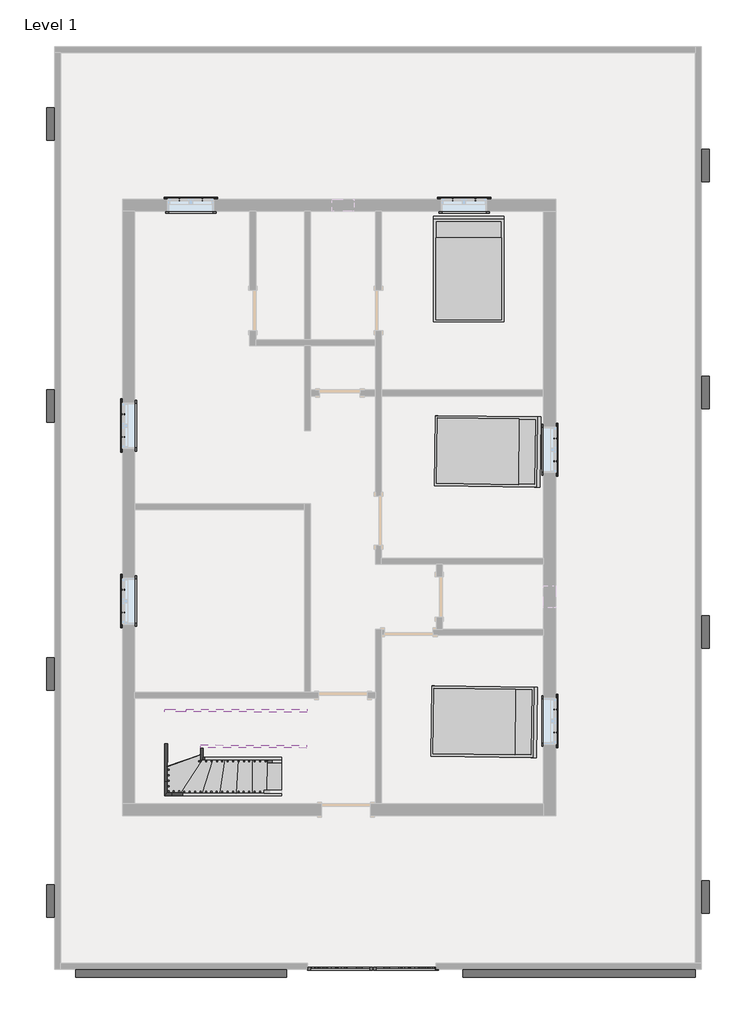
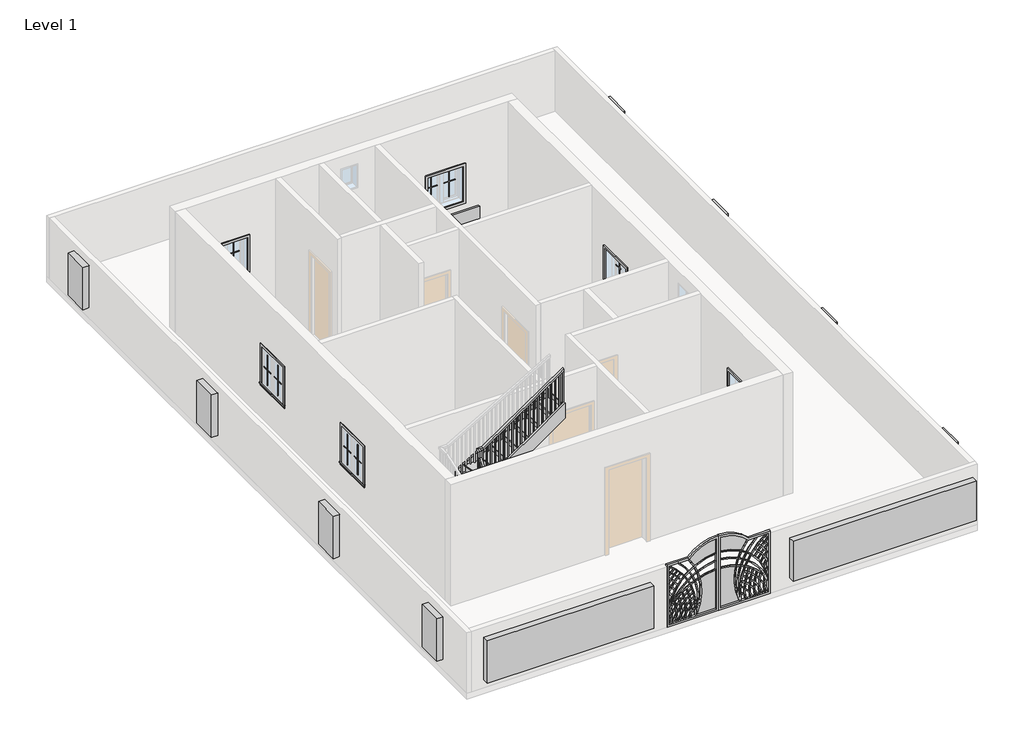
# One storey, part 3 of 3: 28 proxies, 9 members, 3 furniture elements, 1 railing, 1 stair flight.
"""IFC4 building model written with IfcOpenShell, lengths in millimetres."""

from ifc_helpers import new_model, si_unit, frame, origin, place, context, project, spatial, polyline, outline, extrude, faceted_brep, transform, mapped, element, save
from components import generic_models_6bc30956, generic_models_1_generic_models_1_75855b24, generic_models_2_generic_models_2_0c6c8571, generic_models_3_generic_models_3_96fd7fd6, muntin_pattern_2x2_muntin_pattern_2x2_b3fe6957, muntin_pattern_2x2_muntin_pattern_2x2_3e0ecaf2, trim_window_exterior_flat_with_sill_41619996, trim_window_interior_flat_picture_frame_51c85655, bed_17739_bed_17739_15c61121, stair_flight_0ba6b5c4

model = new_model("IFC4")

# Units and contexts
model_context = context("Model", 3, world=origin())
ifc_project = project(units=[si_unit("LENGTHUNIT", "METRE", prefix="MILLI")], contexts=[model_context])

# Site, building, storey
site = spatial("IfcSite", under=ifc_project)
building = spatial("IfcBuilding", under=site)
storey = spatial("IfcBuildingStorey", under=building, Name="Level 1", Elevation=0.0)

# Proxies
placement = place(None, origin())
generic_models_shape = generic_models_6bc30956(model_context)
element("IfcBuildingElementProxy", 1, Name="Generic Models", at=placement, inside=storey, context=model_context, shape_type="MappedRepresentation", body=[
    mapped(generic_models_shape, transform((-629.6367314, -8096.8061589, 0.0), x_axis=(1.0, 0.0, 0.0), y_axis=(0.0, 1.0, 0.0), z_axis=(0.0, 0.0, 1.0))),
])
generic_models_1_generic_models_1_shape = generic_models_1_generic_models_1_75855b24(model_context)
element("IfcBuildingElementProxy", 2, Name="Generic Models 1 : Generic Models 1", ObjectType="Generic Models 1 : Generic Models 1", at=placement, inside=storey, context=model_context, shape_type="MappedRepresentation", body=[
    mapped(generic_models_1_generic_models_1_shape, transform((0.0, 0.0, 0.0), x_axis=(1.0, 0.0, 0.0), y_axis=(0.0, 1.0, 0.0), z_axis=(0.0, 0.0, 1.0))),
])
generic_models_2_generic_models_2_shape = generic_models_2_generic_models_2_0c6c8571(model_context)
element("IfcBuildingElementProxy", 3, Name="Generic Models 2 : Generic Models 2", ObjectType="Generic Models 2 : Generic Models 2", at=placement, inside=storey, context=model_context, shape_type="MappedRepresentation", body=[
    mapped(generic_models_2_generic_models_2_shape, transform((0.0, 0.0, 0.0), x_axis=(1.0, 0.0, 0.0), y_axis=(0.0, 1.0, 0.0), z_axis=(0.0, 0.0, 1.0))),
])
generic_models_3_generic_models_3_shape = generic_models_3_generic_models_3_96fd7fd6(model_context)
element("IfcBuildingElementProxy", 4, Name="Generic Models 3 : Generic Models 3", ObjectType="Generic Models 3 : Generic Models 3", at=placement, inside=storey, context=model_context, shape_type="MappedRepresentation", body=[
    mapped(generic_models_3_generic_models_3_shape, transform((0.0, 0.0, 0.0), x_axis=(1.0, 0.0, 0.0), y_axis=(0.0, 1.0, 0.0), z_axis=(0.0, 0.0, 1.0))),
])
muntin_pattern_2x2_muntin_pattern_2x2_shape = muntin_pattern_2x2_muntin_pattern_2x2_b3fe6957(model_context)
element("IfcBuildingElementProxy", 5, Name="Muntin Pattern_2x2 : Muntin Pattern_2x2", ObjectType="Muntin Pattern_2x2 : Muntin Pattern_2x2", at=placement, inside=storey, context=model_context, shape_type="MappedRepresentation", body=[
    mapped(muntin_pattern_2x2_muntin_pattern_2x2_shape, transform((873.7257686, 6321.6571212, 984.25), x_axis=(1.0, 0.0, 0.0), y_axis=(0.0, 1.0, 0.0), z_axis=(0.0, 0.0, 1.0))),
])
element("IfcBuildingElementProxy", 6, Name="Muntin Pattern_2x2 : Muntin Pattern_2x2", ObjectType="Muntin Pattern_2x2 : Muntin Pattern_2x2", at=placement, inside=storey, context=model_context, shape_type="MappedRepresentation", body=[
    mapped(muntin_pattern_2x2_muntin_pattern_2x2_shape, transform((2802.5382686, 1840.1446212, 984.25), x_axis=(0.0, -1.0, 0.0), y_axis=(1.0, 0.0, 0.0), z_axis=(0.0, 0.0, 1.0))),
])
element("IfcBuildingElementProxy", 7, Name="Muntin Pattern_2x2 : Muntin Pattern_2x2", ObjectType="Muntin Pattern_2x2 : Muntin Pattern_2x2", at=placement, inside=storey, context=model_context, shape_type="MappedRepresentation", body=[
    mapped(muntin_pattern_2x2_muntin_pattern_2x2_shape, transform((2802.5382686, -3255.7303788, 984.25), x_axis=(0.0, -1.0, 0.0), y_axis=(1.0, 0.0, 0.0), z_axis=(0.0, 0.0, 1.0))),
])
element("IfcBuildingElementProxy", 8, Name="Muntin Pattern_2x2 : Muntin Pattern_2x2", ObjectType="Muntin Pattern_2x2 : Muntin Pattern_2x2", at=placement, inside=storey, context=model_context, shape_type="MappedRepresentation", body=[
    mapped(muntin_pattern_2x2_muntin_pattern_2x2_shape, transform((-4263.4242314, 6321.6571212, 984.25), x_axis=(1.0, 0.0, 0.0), y_axis=(0.0, 1.0, 0.0), z_axis=(0.0, 0.0, 1.0))),
])
element("IfcBuildingElementProxy", 9, Name="Muntin Pattern_2x2 : Muntin Pattern_2x2", ObjectType="Muntin Pattern_2x2 : Muntin Pattern_2x2", at=placement, inside=storey, context=model_context, shape_type="MappedRepresentation", body=[
    mapped(muntin_pattern_2x2_muntin_pattern_2x2_shape, transform((-5319.1117314, 1863.8332318, 984.25), x_axis=(0.0, 1.0, 0.0), y_axis=(-1.0, 0.0, 0.0), z_axis=(0.0, 0.0, 1.0))),
])
element("IfcBuildingElementProxy", 10, Name="Muntin Pattern_2x2 : Muntin Pattern_2x2", ObjectType="Muntin Pattern_2x2 : Muntin Pattern_2x2", at=placement, inside=storey, context=model_context, shape_type="MappedRepresentation", body=[
    mapped(muntin_pattern_2x2_muntin_pattern_2x2_shape, transform((-5319.1117314, -1431.8167682, 984.25), x_axis=(0.0, 1.0, 0.0), y_axis=(-1.0, 0.0, 0.0), z_axis=(0.0, 0.0, 1.0))),
])
muntin_pattern_2x2_muntin_pattern_2x2_2_shape = muntin_pattern_2x2_muntin_pattern_2x2_3e0ecaf2(model_context)
element("IfcBuildingElementProxy", 11, Name="Muntin Pattern_2x2 : Muntin Pattern_2x2", ObjectType="Muntin Pattern_2x2 : Muntin Pattern_2x2", at=placement, inside=storey, context=model_context, shape_type="MappedRepresentation", body=[
    mapped(muntin_pattern_2x2_muntin_pattern_2x2_2_shape, transform((1302.3507686, 6321.6571212, 984.25), x_axis=(-1.0, 0.0, 0.0), y_axis=(0.0, -1.0, 0.0), z_axis=(0.0, 0.0, 1.0))),
])
element("IfcBuildingElementProxy", 12, Name="Muntin Pattern_2x2 : Muntin Pattern_2x2", ObjectType="Muntin Pattern_2x2 : Muntin Pattern_2x2", at=placement, inside=storey, context=model_context, shape_type="MappedRepresentation", body=[
    mapped(muntin_pattern_2x2_muntin_pattern_2x2_2_shape, transform((2802.5382686, 1411.5196212, 984.25), x_axis=(0.0, 1.0, 0.0), y_axis=(-1.0, 0.0, 0.0), z_axis=(0.0, 0.0, 1.0))),
])
element("IfcBuildingElementProxy", 13, Name="Muntin Pattern_2x2 : Muntin Pattern_2x2", ObjectType="Muntin Pattern_2x2 : Muntin Pattern_2x2", at=placement, inside=storey, context=model_context, shape_type="MappedRepresentation", body=[
    mapped(muntin_pattern_2x2_muntin_pattern_2x2_2_shape, transform((2802.5382686, -3684.3553788, 984.25), x_axis=(0.0, 1.0, 0.0), y_axis=(-1.0, 0.0, 0.0), z_axis=(0.0, 0.0, 1.0))),
])
element("IfcBuildingElementProxy", 14, Name="Muntin Pattern_2x2 : Muntin Pattern_2x2", ObjectType="Muntin Pattern_2x2 : Muntin Pattern_2x2", at=placement, inside=storey, context=model_context, shape_type="MappedRepresentation", body=[
    mapped(muntin_pattern_2x2_muntin_pattern_2x2_2_shape, transform((-3834.7992314, 6321.6571212, 984.25), x_axis=(-1.0, 0.0, 0.0), y_axis=(0.0, -1.0, 0.0), z_axis=(0.0, 0.0, 1.0))),
])
element("IfcBuildingElementProxy", 15, Name="Muntin Pattern_2x2 : Muntin Pattern_2x2", ObjectType="Muntin Pattern_2x2 : Muntin Pattern_2x2", at=placement, inside=storey, context=model_context, shape_type="MappedRepresentation", body=[
    mapped(muntin_pattern_2x2_muntin_pattern_2x2_2_shape, transform((-5319.1117314, 2292.4582318, 984.25), x_axis=(0.0, -1.0, 0.0), y_axis=(1.0, 0.0, 0.0), z_axis=(0.0, 0.0, 1.0))),
])
element("IfcBuildingElementProxy", 16, Name="Muntin Pattern_2x2 : Muntin Pattern_2x2", ObjectType="Muntin Pattern_2x2 : Muntin Pattern_2x2", at=placement, inside=storey, context=model_context, shape_type="MappedRepresentation", body=[
    mapped(muntin_pattern_2x2_muntin_pattern_2x2_2_shape, transform((-5319.1117314, -1003.1917682, 984.25), x_axis=(0.0, -1.0, 0.0), y_axis=(1.0, 0.0, 0.0), z_axis=(0.0, 0.0, 1.0))),
])
trim_window_exterior_flat_with_sill_shape = trim_window_exterior_flat_with_sill_41619996(model_context)
element("IfcBuildingElementProxy", 17, Name="Trim-Window-Exterior-Flat : with Sill", ObjectType="Trim-Window-Exterior-Flat : with Sill", at=placement, inside=storey, context=model_context, shape_type="MappedRepresentation", body=[
    mapped(trim_window_exterior_flat_with_sill_shape, transform((1088.0382686, 6331.1821212, 1828.8), x_axis=(-1.0, 0.0, 0.0), y_axis=(0.0, 0.0, 1.0), z_axis=(0.0, 1.0, 0.0))),
])
element("IfcBuildingElementProxy", 18, Name="Trim-Window-Exterior-Flat : with Sill", ObjectType="Trim-Window-Exterior-Flat : with Sill", at=placement, inside=storey, context=model_context, shape_type="MappedRepresentation", body=[
    mapped(trim_window_exterior_flat_with_sill_shape, transform((2812.0632686, 1625.8321212, 1828.8), x_axis=(0.0, 1.0, 0.0), y_axis=(0.0, 0.0, 1.0), z_axis=(1.0, 0.0, 0.0))),
])
element("IfcBuildingElementProxy", 19, Name="Trim-Window-Exterior-Flat : with Sill", ObjectType="Trim-Window-Exterior-Flat : with Sill", at=placement, inside=storey, context=model_context, shape_type="MappedRepresentation", body=[
    mapped(trim_window_exterior_flat_with_sill_shape, transform((2812.0632686, -3470.0428788, 1828.8), x_axis=(0.0, 1.0, 0.0), y_axis=(0.0, 0.0, 1.0), z_axis=(1.0, 0.0, 0.0))),
])
element("IfcBuildingElementProxy", 20, Name="Trim-Window-Exterior-Flat : with Sill", ObjectType="Trim-Window-Exterior-Flat : with Sill", at=placement, inside=storey, context=model_context, shape_type="MappedRepresentation", body=[
    mapped(trim_window_exterior_flat_with_sill_shape, transform((-4049.1117314, 6331.1821212, 1828.8), x_axis=(-1.0, 0.0, 0.0), y_axis=(0.0, 0.0, 1.0), z_axis=(0.0, 1.0, 0.0))),
])
element("IfcBuildingElementProxy", 21, Name="Trim-Window-Exterior-Flat : with Sill", ObjectType="Trim-Window-Exterior-Flat : with Sill", at=placement, inside=storey, context=model_context, shape_type="MappedRepresentation", body=[
    mapped(trim_window_exterior_flat_with_sill_shape, transform((-5328.6367314, 2078.1457318, 1828.8), x_axis=(0.0, -1.0, 0.0), y_axis=(0.0, 0.0, 1.0), z_axis=(-1.0, 0.0, 0.0))),
])
element("IfcBuildingElementProxy", 22, Name="Trim-Window-Exterior-Flat : with Sill", ObjectType="Trim-Window-Exterior-Flat : with Sill", at=placement, inside=storey, context=model_context, shape_type="MappedRepresentation", body=[
    mapped(trim_window_exterior_flat_with_sill_shape, transform((-5328.6367314, -1217.5042682, 1828.8), x_axis=(0.0, -1.0, 0.0), y_axis=(0.0, 0.0, 1.0), z_axis=(-1.0, 0.0, 0.0))),
])
trim_window_interior_flat_picture_frame_shape = trim_window_interior_flat_picture_frame_51c85655(model_context)
element("IfcBuildingElementProxy", 23, Name="Trim-Window-Interior-Flat : Picture Frame", ObjectType="Trim-Window-Interior-Flat : Picture Frame", at=placement, inside=storey, context=model_context, shape_type="MappedRepresentation", body=[
    mapped(trim_window_interior_flat_picture_frame_shape, transform((1088.0382686, 6102.5821212, 1828.8), x_axis=(1.0, 0.0, 0.0), y_axis=(0.0, 0.0, 1.0), z_axis=(0.0, -1.0, 0.0))),
])
element("IfcBuildingElementProxy", 24, Name="Trim-Window-Interior-Flat : Picture Frame", ObjectType="Trim-Window-Interior-Flat : Picture Frame", at=placement, inside=storey, context=model_context, shape_type="MappedRepresentation", body=[
    mapped(trim_window_interior_flat_picture_frame_shape, transform((2583.4632686, 1625.8321212, 1828.8), x_axis=(0.0, -1.0, 0.0), y_axis=(0.0, 0.0, 1.0), z_axis=(-1.0, 0.0, 0.0))),
])
element("IfcBuildingElementProxy", 25, Name="Trim-Window-Interior-Flat : Picture Frame", ObjectType="Trim-Window-Interior-Flat : Picture Frame", at=placement, inside=storey, context=model_context, shape_type="MappedRepresentation", body=[
    mapped(trim_window_interior_flat_picture_frame_shape, transform((2583.4632686, -3470.0428788, 1828.8), x_axis=(0.0, -1.0, 0.0), y_axis=(0.0, 0.0, 1.0), z_axis=(-1.0, 0.0, 0.0))),
])
element("IfcBuildingElementProxy", 26, Name="Trim-Window-Interior-Flat : Picture Frame", ObjectType="Trim-Window-Interior-Flat : Picture Frame", at=placement, inside=storey, context=model_context, shape_type="MappedRepresentation", body=[
    mapped(trim_window_interior_flat_picture_frame_shape, transform((-4049.1117314, 6102.5821212, 1828.8), x_axis=(1.0, 0.0, 0.0), y_axis=(0.0, 0.0, 1.0), z_axis=(0.0, -1.0, 0.0))),
])
element("IfcBuildingElementProxy", 27, Name="Trim-Window-Interior-Flat : Picture Frame", ObjectType="Trim-Window-Interior-Flat : Picture Frame", at=placement, inside=storey, context=model_context, shape_type="MappedRepresentation", body=[
    mapped(trim_window_interior_flat_picture_frame_shape, transform((-5100.0367314, 2078.1457318, 1828.8), x_axis=(0.0, 1.0, 0.0), y_axis=(0.0, 0.0, 1.0), z_axis=(1.0, 0.0, 0.0))),
])
element("IfcBuildingElementProxy", 28, Name="Trim-Window-Interior-Flat : Picture Frame", ObjectType="Trim-Window-Interior-Flat : Picture Frame", at=placement, inside=storey, context=model_context, shape_type="MappedRepresentation", body=[
    mapped(trim_window_interior_flat_picture_frame_shape, transform((-5100.0367314, -1217.5042682, 1828.8), x_axis=(0.0, 1.0, 0.0), y_axis=(0.0, 0.0, 1.0), z_axis=(1.0, 0.0, 0.0))),
])

# Furniture
bed_17739_bed_17739_shape = bed_17739_bed_17739_15c61121(model_context)
element("IfcFurniture", 29, ObjectType="Bed_17739 : Bed_17739", at=placement, inside=storey, context=model_context, shape_type="MappedRepresentation", body=[
    mapped(bed_17739_bed_17739_shape, transform((1173.7632686, 4997.6821212, 0.0), x_axis=(1.0, 0.0, 0.0), y_axis=(0.0, 1.0, 0.0), z_axis=(0.0, 0.0, 1.0))),
])
element("IfcFurniture", 30, ObjectType="Bed_17739 : Bed_17739", at=placement, inside=storey, context=model_context, shape_type="MappedRepresentation", body=[
    mapped(bed_17739_bed_17739_shape, transform((1503.3372561, 1596.4447738, 0.0), x_axis=(-0.012740965827000846, -0.9999188306006619, 0.0), y_axis=(0.9999188306006619, -0.012740965827000846, 0.0), z_axis=(0.0, 0.0, 1.0))),
])
element("IfcFurniture", 31, ObjectType="Bed_17739 : Bed_17739", at=placement, inside=storey, context=model_context, shape_type="MappedRepresentation", body=[
    mapped(bed_17739_bed_17739_shape, transform((1438.6034215, -3483.9063624, 0.0), x_axis=(-0.012740965827007402, -0.9999188306006618, 0.0), y_axis=(0.9999188306006618, -0.012740965827007402, 0.0), z_axis=(0.0, 0.0, 1.0))),
])

# Members
element("IfcMember", 32, ObjectType="Stringer - 2\" Width", at=placement, inside=storey, context=model_context, shape_type="SweptSolid", body=[
    extrude(outline(polyline([(-105.6436802, -202.41926), (0.0, 0.0), (2328.0658822, 0.0), (2168.9891534, -304.7999999), (90.5236019, -304.7999999), (-105.6436802, -202.41926)])), frame((-2342.1993001, -4876.8012848, 228.3290257), z_axis=(0.003383581801438567, 0.9999942756707125, 0.0), x_axis=(-0.8865193579369284, 0.002999627936996438, 0.46268178074713073)), (0.0, 0.0, 1.0), 50.8),
])
element("IfcMember", 33, ObjectType="Stringer - 2\" Width", at=placement, inside=storey, context=model_context, shape_type="SweptSolid", body=[
    extrude(outline(polyline([(-4405.9028852, -4819.0182441), (-4406.0747712, -4869.8179533), (-4542.6986856, -4869.3556725), (-4491.7270905, -4818.7278493), (-4405.9028852, -4819.0182441)])), frame((0.0, 0.0, 961.6681426), z_axis=(0.0, 0.0, 1.0), x_axis=(1.0, 0.0, 0.0)), (0.0, 0.0, 1.0), 343.8145513),
])
element("IfcMember", 34, ObjectType="Stringer - 2\" Width", at=placement, inside=storey, context=model_context, shape_type="SweptSolid", body=[
    extrude(outline(polyline([(-4491.7270905, -4818.7278493), (-4542.6986856, -4869.3556725), (-4541.8102896, -4606.7963526), (-4491.0105804, -4606.9682386), (-4491.7270905, -4818.7278493)])), frame((0.0, 0.0, 961.6681426), z_axis=(0.0, 0.0, 1.0), x_axis=(1.0, 0.0, 0.0)), (0.0, 0.0, 1.0), 343.8145513),
])
element("IfcMember", 35, ObjectType="Stringer - 2\" Width", at=placement, inside=storey, context=model_context, shape_type="SweptSolid", body=[
    extrude(outline(polyline([(109.7110974, -325.8403301), (0.0, 0.0), (1383.9510961, 0.0), (1489.930143, -314.7561954), (1457.0104275, -325.8403301), (109.7110974, -325.8403301)])), frame((-4491.0105804, -4606.9682386, 961.6681426), z_axis=(-0.9999942756707125, 0.003383581801438886, 0.0), x_axis=(0.0032066921171017464, 0.9477157489074122, 0.3190996339680271)), (0.0, 0.0, 1.0), 50.8),
])
element("IfcMember", 36, ObjectType="Stringer - 2\" Width", at=placement, inside=storey, context=model_context, shape_type="SweptSolid", body=[
    extrude(outline(polyline([(-4537.3723845, -3295.2041032), (-4537.2004986, -3244.404394), (-4139.0142012, -3245.7516976), (-4139.1860871, -3296.5514068), (-4537.3723845, -3295.2041032)])), frame((0.0, 0.0, 1413.7918365), z_axis=(0.0, 0.0, 1.0), x_axis=(1.0, 0.0, 0.0)), (0.0, 0.0, 1.0), 321.6135804),
])
element("IfcMember", 37, ObjectType="Stringer - 2\" Width", at=placement, inside=storey, context=model_context, shape_type="SweptSolid", body=[
    extrude(outline(polyline([(-111.9549294, -160.635527), (0.0, 0.0), (1800.2454177, 0.0), (1587.8150598, -304.8000001), (94.8955973, -304.8), (-111.9549294, -160.635527)])), frame((-2339.9228929, -4204.0248458, 195.8000989), z_axis=(0.0033835818014388334, 0.9999942756707125, 0.0), x_axis=(-0.8204010535979693, 0.002775909965058046, 0.5717817814334486)), (0.0, 0.0, 1.0), 50.8),
])
element("IfcMember", 38, ObjectType="Stringer - 2\" Width", at=placement, inside=storey, context=model_context, shape_type="SweptSolid", body=[
    extrude(outline(polyline([(438.5777673, -304.8), (2.5808594, -1.7936294), (3.8273846, 0.0), (400.5684618, 0.0), (819.8223258, -291.370396), (810.4891046, -304.8000001), (438.5777673, -304.8)])), frame((-3816.8461303, -4199.0275266, 885.8862902), z_axis=(-0.9999942756707125, 0.003383581801437359, 0.0), x_axis=(0.0019309727886812915, 0.5706856959500503, 0.8211663094538744)), (0.0, 0.0, 1.0), 50.8),
])
element("IfcMember", 39, ObjectType="Stringer - 2\" Width", at=placement, inside=storey, context=model_context, shape_type="SweptSolid", body=[
    extrude(outline(polyline([(213.8292849, -304.8), (0.0, 0.0), (2440.5867528, 0.0), (2654.4160377, -304.8), (213.8292849, -304.8)])), frame((-3866.8723527, -3970.2569493, 1353.0535021), z_axis=(0.003383581801438697, 0.9999942756707126, 0.0), x_axis=(0.8186346554264394, -0.0027699331781375547, 0.5743079560697585)), (0.0, 0.0, 1.0), 50.8),
])
element("IfcMember", 40, ObjectType="Stringer - 2\" Width", at=placement, inside=storey, context=model_context, shape_type="SweptSolid", body=[
    extrude(outline(polyline([(162.5062199, -277.5374274), (0.0, 0.0), (2633.4595913, 1e-07), (2795.9658112, -277.5374274), (162.5062199, -277.5374274)])), frame((-4139.1860871, -3296.5514068, 1413.7918365), z_axis=(0.0033835818014385914, 0.9999942756707125, 0.0), x_axis=(0.8629481327443969, -0.002919872311849945, 0.5052840731100093)), (0.0, 0.0, 1.0), 50.8),
])

# Railing
element("IfcRailing", 41, ObjectType="Handrail - Rectangular", at=placement, inside=storey, context=model_context, shape_type="SolidModel", body=[
    faceted_brep([(-2340.0947789, -4254.824555, 1083.7333333), (-2340.0947789, -4254.824555, 1022.3023206), (-2339.9228929, -4204.0248458, 1022.3023206), (-2339.9228929, -4204.0248458, 1083.7333333), (-3791.6181617, -4249.9131788, 2070.7092848), (-3842.4178709, -4249.7412929, 2043.8199762), (-3842.2459849, -4198.9415837, 2043.8199762), (-3791.4462757, -4199.1134696, 2070.7092848), (-1868.5796854, -3875.4177931, 3962.4), (-1868.7515713, -3926.2175023, 3962.4), (-1868.7515713, -3926.2175023, 3900.738507), (-1868.5796854, -3875.4177931, 3900.738507), (-3774.5418549, -3868.9687773, 2589.445528), (-3790.329017, -3868.9153598, 2640.245528), (-3774.7137409, -3919.7684865, 2589.445528), (-3790.500903, -3919.715069, 2640.245528), (-3791.6181617, -4249.9131788, 2287.0182666), (-3842.4178709, -4249.7412929, 2236.2182666), (-3842.2459849, -4198.9415837, 2236.2182666), (-3791.4462757, -4199.1134696, 2287.0182666), (-3918.6174347, -4249.4834639, 2287.0182666), (-3918.6174347, -4249.4834639, 2236.2182666), (-3867.6458395, -4198.8556407, 2236.2182666), (-3867.6458395, -4198.8556407, 2287.0182666), (-3918.1877198, -4122.4841909, 2287.0182666), (-3918.0978567, -4095.9257757, 2236.2182666), (-3867.2981475, -4096.0976616, 2236.2182666), (-3867.3880106, -4122.6560769, 2287.0182666), (-3917.7580049, -3995.4849179, 2469.759003), (-3917.586119, -3944.6852087, 2453.8400838), (-3866.7864097, -3944.8570947, 2453.8400838), (-3866.9582957, -3995.6568039, 2469.759003), (-3917.7580049, -3995.4849179, 2640.245528), (-3917.586119, -3944.6852087, 2589.445528), (-3866.7864097, -3944.8570947, 2589.445528), (-3866.9582957, -3995.6568039, 2640.245528), (-3917.32829, -3868.4856449, 2640.245528), (-3917.32829, -3868.4856449, 2589.445528), (-3866.7004668, -3919.4572401, 2589.445528), (-3866.7004668, -3919.4572401, 2640.245528)], [[[0, 1, 2, 3]], [[1, 0, 4, 5]], [[2, 1, 5, 6]], [[3, 2, 6, 7]], [[0, 3, 7, 4]], [[8, 9, 10, 11]], [[12, 13, 8, 11]], [[14, 12, 11, 10]], [[15, 14, 10, 9]], [[13, 15, 9, 8]], [[5, 4, 16, 17]], [[6, 5, 17, 18]], [[7, 6, 18, 19]], [[4, 7, 19, 16]], [[17, 16, 20, 21]], [[18, 17, 21, 22]], [[19, 18, 22, 23]], [[16, 19, 23, 20]], [[21, 20, 24, 25]], [[22, 21, 25, 26]], [[23, 22, 26, 27]], [[20, 23, 27, 24]], [[25, 24, 28, 29]], [[26, 25, 29, 30]], [[27, 26, 30, 31]], [[24, 27, 31, 28]], [[29, 28, 32, 33]], [[30, 29, 33, 34]], [[31, 30, 34, 35]], [[28, 31, 35, 32]], [[33, 32, 36, 37]], [[34, 33, 37, 38]], [[35, 34, 38, 39]], [[32, 35, 39, 36]], [[37, 36, 13, 12]], [[38, 37, 12, 14]], [[39, 38, 14, 15]], [[36, 39, 15, 13]]]),
    extrude(outline(polyline([(222.0468824, -19.0499999), (235.1531175, 0.0), (1186.7159363, 0.0), (1186.7159363, -19.0499999), (222.0468824, -19.0499999)])), frame((-1971.1826027, -3909.9958257, 4065.382603), z_axis=(0.0033835818014386967, 0.9999942756707125, 0.0), x_axis=(0.0, 0.0, -1.0)), (0.0, 0.0, 1.0), 19.05),
    extrude(outline(polyline([(222.0468825, -19.0499999), (235.1531175, 0.0), (1116.8160159, 0.0), (1116.8160159, -19.0499999), (222.0468825, -19.0499999)])), frame((-2072.7820211, -3909.6520537, 3995.4826826), z_axis=(0.0033835818014386967, 0.9999942756707125, 0.0), x_axis=(0.0, 0.0, -1.0)), (0.0, 0.0, 1.0), 19.05),
    extrude(outline(polyline([(222.0468825, -19.0499999), (235.1531176, 0.0), (1216.2494289, 0.0), (1216.2494289, -19.0499999), (222.0468825, -19.0499999)])), frame((-2174.3814395, -3909.3082818, 3925.5827622), z_axis=(0.0033835818014386967, 0.9999942756707125, 0.0), x_axis=(0.0, 0.0, -1.0)), (0.0, 0.0, 1.0), 19.05),
    extrude(outline(polyline([(222.0468825, -19.05), (235.1531175, 0.0), (1146.3495084, 0.0), (1146.3495084, -19.05), (222.0468825, -19.05)])), frame((-2275.980858, -3908.9645099, 3855.6828417), z_axis=(0.0033835818014386967, 0.9999942756707125, 0.0), x_axis=(0.0, 0.0, -1.0)), (0.0, 0.0, 1.0), 19.05),
    extrude(outline(polyline([(222.0468825, -19.05), (235.1531176, 0.0), (1076.449588, 0.0), (1076.449588, -19.05), (222.0468825, -19.05)])), frame((-2377.5802764, -3908.620738, 3785.7829213), z_axis=(0.0033835818014386967, 0.9999942756707125, 0.0), x_axis=(0.0, 0.0, -1.0)), (0.0, 0.0, 1.0), 19.05),
    extrude(outline(polyline([(222.0468824, -19.05), (235.1531175, 0.0), (1175.8830008, 0.0), (1175.8830008, -19.05), (222.0468824, -19.05)])), frame((-2479.1796948, -3908.2769661, 3715.8830008), z_axis=(0.0033835818014386967, 0.9999942756707125, 0.0), x_axis=(0.0, 0.0, -1.0)), (0.0, 0.0, 1.0), 19.05),
    extrude(outline(polyline([(222.0468825, -19.05), (235.1531176, 0.0), (1105.9830804, 0.0), (1105.9830804, -19.05), (222.0468825, -19.05)])), frame((-2580.7791132, -3907.9331942, 3645.9830804), z_axis=(0.0033835818014386967, 0.9999942756707125, 0.0), x_axis=(0.0, 0.0, -1.0)), (0.0, 0.0, 1.0), 19.05),
    extrude(outline(polyline([(222.0468824, -19.05), (235.1531175, 0.0), (1036.0831599, 0.0), (1036.0831599, -19.05), (222.0468824, -19.05)])), frame((-2682.3785316, -3907.5894223, 3576.0831599), z_axis=(0.0033835818014386967, 0.9999942756707125, 0.0), x_axis=(0.0, 0.0, -1.0)), (0.0, 0.0, 1.0), 19.05),
    extrude(outline(polyline([(222.0468825, -19.05), (235.1531176, 0.0), (1135.5165728, 0.0), (1135.5165728, -19.05), (222.0468825, -19.05)])), frame((-2783.97795, -3907.2456504, 3506.1832395), z_axis=(0.0033835818014386967, 0.9999942756707125, 0.0), x_axis=(0.0, 0.0, -1.0)), (0.0, 0.0, 1.0), 19.05),
    extrude(outline(polyline([(222.0468824, -19.0499999), (235.1531175, 0.0), (1065.6166523, 0.0), (1065.6166523, -19.0499999), (222.0468824, -19.0499999)])), frame((-2885.5773684, -3906.9018785, 3436.283319), z_axis=(0.0033835818014386967, 0.9999942756707125, 0.0), x_axis=(0.0, 0.0, -1.0)), (0.0, 0.0, 1.0), 19.05),
    extrude(outline(polyline([(222.0468825, -19.0499999), (235.1531176, 0.0), (995.7167319, 0.0), (995.7167319, -19.0499999), (222.0468825, -19.0499999)])), frame((-2987.1767868, -3906.5581065, 3366.3833986), z_axis=(0.0033835818014386967, 0.9999942756707125, 0.0), x_axis=(0.0, 0.0, -1.0)), (0.0, 0.0, 1.0), 19.05),
    extrude(outline(polyline([(222.0468824, -19.0499999), (235.1531175, 0.0), (1095.1501448, 0.0), (1095.1501448, -19.0499999), (222.0468824, -19.0499999)])), frame((-3088.7762052, -3906.2143346, 3296.4834781), z_axis=(0.0033835818014386967, 0.9999942756707125, 0.0), x_axis=(0.0, 0.0, -1.0)), (0.0, 0.0, 1.0), 19.05),
    extrude(outline(polyline([(222.0468825, -19.0499999), (235.1531176, 0.0), (1025.2502244, 0.0), (1025.2502244, -19.0499999), (222.0468825, -19.0499999)])), frame((-3190.3756236, -3905.8705627, 3226.5835577), z_axis=(0.0033835818014386967, 0.9999942756707125, 0.0), x_axis=(0.0, 0.0, -1.0)), (0.0, 0.0, 1.0), 19.05),
    extrude(outline(polyline([(222.0468824, -19.0499999), (235.1531175, 0.0), (1124.6836372, 0.0), (1124.6836372, -19.0499999), (222.0468824, -19.0499999)])), frame((-3291.975042, -3905.5267908, 3156.6836372), z_axis=(0.0033835818014386967, 0.9999942756707125, 0.0), x_axis=(0.0, 0.0, -1.0)), (0.0, 0.0, 1.0), 19.05),
    extrude(outline(polyline([(222.0468825, -19.0499999), (235.1531176, 0.0), (1054.7837168, 0.0), (1054.7837168, -19.0499999), (222.0468825, -19.0499999)])), frame((-3393.5744604, -3905.1830189, 3086.7837168), z_axis=(0.0033835818014386967, 0.9999942756707125, 0.0), x_axis=(0.0, 0.0, -1.0)), (0.0, 0.0, 1.0), 19.05),
    extrude(outline(polyline([(222.0468824, -19.05), (235.1531175, 0.0), (984.8837963, 0.0), (984.8837963, -19.05), (222.0468824, -19.05)])), frame((-3495.1738789, -3904.839247, 3016.8837963), z_axis=(0.0033835818014386967, 0.9999942756707125, 0.0), x_axis=(0.0, 0.0, -1.0)), (0.0, 0.0, 1.0), 19.05),
    extrude(outline(polyline([(222.0468825, -19.05), (235.1531176, 0.0), (1084.3172092, 0.0), (1084.3172092, -19.05), (222.0468825, -19.05)])), frame((-3596.7732973, -3904.4954751, 2946.9838759), z_axis=(0.0033835818014386967, 0.9999942756707125, 0.0), x_axis=(0.0, 0.0, -1.0)), (0.0, 0.0, 1.0), 19.05),
    extrude(outline(polyline([(222.0468824, -19.05), (235.1531175, 0.0), (1014.4172887, 0.0), (1014.4172887, -19.05), (222.0468824, -19.05)])), frame((-3698.3727157, -3904.1517032, 2877.0839554), z_axis=(0.0033835818014386967, 0.9999942756707125, 0.0), x_axis=(0.0, 0.0, -1.0)), (0.0, 0.0, 1.0), 19.05),
    extrude(outline(polyline([(222.0468825, -19.05), (235.1531175, 0.0), (1113.8507017, 0.0), (1113.8507017, -19.05), (222.0468825, -19.05)])), frame((-3799.9721341, -3903.8079313, 2807.184035), z_axis=(0.0033835818014386967, 0.9999942756707125, 0.0), x_axis=(0.0, 0.0, -1.0)), (0.0, 0.0, 1.0), 19.05),
    extrude(outline(polyline([(-3882.6076045, -3928.9284712), (-3901.6574955, -3928.8640139), (-3901.5930382, -3909.814123), (-3882.5431473, -3909.8785802), (-3882.6076045, -3928.9284712)])), frame((0.0, 0.0, 1524.0), z_axis=(0.0, 0.0, 1.0), x_axis=(1.0, 0.0, 0.0)), (0.0, 0.0, 1.0), 1065.445528),
    extrude(outline(polyline([(214.8944448, -19.05), (242.3055552, 0.0), (1218.1289753, 0.0), (1218.1289753, -19.05), (214.8944448, -19.05)])), frame((-3882.9513764, -4030.5278896, 2572.795642), z_axis=(-0.9999942756707125, 0.0033835818014373593, 0.0), x_axis=(0.0, 0.0, -1.0)), (0.0, 0.0, 1.0), 19.05),
    extrude(outline(polyline([(214.8944448, -19.05), (242.3055552, 0.0), (1071.9363862, 0.0), (1071.9363862, -19.05), (214.8944448, -19.05)])), frame((-3883.2951483, -4132.127308, 2426.6030529), z_axis=(-0.9999942756707125, 0.0033835818014373593, 0.0), x_axis=(0.0, 0.0, -1.0)), (0.0, 0.0, 1.0), 19.05),
    extrude(outline(polyline([(-3854.4429379, -4214.7754049), (-3854.5073951, -4233.8252959), (-3873.5572861, -4233.7608386), (-3873.4928289, -4214.7109477), (-3854.4429379, -4214.7754049)])), frame((0.0, 0.0, 1185.3333333), z_axis=(0.0, 0.0, 1.0), x_axis=(1.0, 0.0, 0.0)), (0.0, 0.0, 1.0), 1050.8849333),
    extrude(outline(polyline([(235.0765695, -19.05), (222.1234305, 0.0), (1202.0700381, 0.0), (1202.0700381, -19.05), (235.0765695, -19.05)])), frame((-3771.9578677, -4234.1046105, 2218.0700381), z_axis=(0.003383581801438833, 0.9999942756707125, 0.0), x_axis=(0.0, 0.0, -1.0)), (0.0, 0.0, 1.0), 19.05),
    extrude(outline(polyline([(235.0765695, -19.05), (222.1234305, 0.0), (1132.9866297, 0.0), (1132.9866297, -19.05), (235.0765695, -19.05)])), frame((-3670.3584493, -4234.4483825, 2148.9866297), z_axis=(0.003383581801438833, 0.9999942756707125, 0.0), x_axis=(0.0, 0.0, -1.0)), (0.0, 0.0, 1.0), 19.05),
    extrude(outline(polyline([(235.0765695, -19.05), (222.1234305, 0.0), (1233.2365546, 0.0), (1233.2365546, -19.05), (235.0765695, -19.05)])), frame((-3568.7590309, -4234.7921544, 2079.9032213), z_axis=(0.003383581801438833, 0.9999942756707125, 0.0), x_axis=(0.0, 0.0, -1.0)), (0.0, 0.0, 1.0), 19.05),
    extrude(outline(polyline([(235.0765695, -19.05), (222.1234305, 0.0), (1164.1531462, 0.0), (1164.1531462, -19.05), (235.0765695, -19.05)])), frame((-3467.1596125, -4235.1359263, 2010.8198129), z_axis=(0.003383581801438833, 0.9999942756707125, 0.0), x_axis=(0.0, 0.0, -1.0)), (0.0, 0.0, 1.0), 19.05),
    extrude(outline(polyline([(235.0765695, -19.05), (222.1234305, 0.0), (1264.4030712, 0.0), (1264.4030712, -19.05), (235.0765695, -19.05)])), frame((-3365.5601941, -4235.4796982, 1941.7364045), z_axis=(0.003383581801438833, 0.9999942756707125, 0.0), x_axis=(0.0, 0.0, -1.0)), (0.0, 0.0, 1.0), 19.05),
    extrude(outline(polyline([(235.0765695, -19.0499999), (222.1234304, 0.0), (1195.3196628, 0.0), (1195.3196628, -19.0499999), (235.0765695, -19.0499999)])), frame((-3263.9607756, -4235.8234701, 1872.6529961), z_axis=(0.003383581801438833, 0.9999942756707125, 0.0), x_axis=(0.0, 0.0, -1.0)), (0.0, 0.0, 1.0), 19.05),
    extrude(outline(polyline([(235.0765695, -19.0499999), (222.1234304, 0.0), (1295.5695877, 0.0), (1295.5695877, -19.0499999), (235.0765695, -19.0499999)])), frame((-3162.3613572, -4236.167242, 1803.5695877), z_axis=(0.003383581801438833, 0.9999942756707125, 0.0), x_axis=(0.0, 0.0, -1.0)), (0.0, 0.0, 1.0), 19.05),
    extrude(outline(polyline([(235.0765695, -19.0499999), (222.1234304, 0.0), (1226.4861793, 0.0), (1226.4861793, -19.0499999), (235.0765695, -19.0499999)])), frame((-3060.7619388, -4236.5110139, 1734.4861793), z_axis=(0.003383581801438833, 0.9999942756707125, 0.0), x_axis=(0.0, 0.0, -1.0)), (0.0, 0.0, 1.0), 19.05),
    extrude(outline(polyline([(235.0765695, -19.0499999), (222.1234304, 0.0), (1157.4027709, 0.0), (1157.4027709, -19.0499999), (235.0765695, -19.0499999)])), frame((-2959.1625204, -4236.8547858, 1665.4027709), z_axis=(0.003383581801438833, 0.9999942756707125, 0.0), x_axis=(0.0, 0.0, -1.0)), (0.0, 0.0, 1.0), 19.05),
    extrude(outline(polyline([(235.0765695, -19.0499999), (222.1234304, 0.0), (1257.6526958, 0.0), (1257.6526958, -19.0499999), (235.0765695, -19.0499999)])), frame((-2857.563102, -4237.1985577, 1596.3193625), z_axis=(0.003383581801438833, 0.9999942756707125, 0.0), x_axis=(0.0, 0.0, -1.0)), (0.0, 0.0, 1.0), 19.05),
    extrude(outline(polyline([(235.0765695, -19.0499999), (222.1234304, 0.0), (1188.5692874, 0.0), (1188.5692874, -19.0499999), (235.0765695, -19.0499999)])), frame((-2755.9636836, -4237.5423297, 1527.2359541), z_axis=(0.003383581801438833, 0.9999942756707125, 0.0), x_axis=(0.0, 0.0, -1.0)), (0.0, 0.0, 1.0), 19.05),
    extrude(outline(polyline([(235.0765696, -19.05), (222.1234305, 0.0), (1119.4858791, 0.0), (1119.4858791, -19.05), (235.0765696, -19.05)])), frame((-2654.3642652, -4237.8861016, 1458.1525458), z_axis=(0.003383581801438833, 0.9999942756707125, 0.0), x_axis=(0.0, 0.0, -1.0)), (0.0, 0.0, 1.0), 19.05),
    extrude(outline(polyline([(235.0765696, -19.05), (222.1234305, 0.0), (1219.7358041, 0.0), (1219.7358041, -19.05), (235.0765696, -19.05)])), frame((-2552.7648468, -4238.2298735, 1389.0691374), z_axis=(0.003383581801438833, 0.9999942756707125, 0.0), x_axis=(0.0, 0.0, -1.0)), (0.0, 0.0, 1.0), 19.05),
    extrude(outline(polyline([(235.0765696, -19.05), (222.1234305, 0.0), (1150.6523957, 0.0), (1150.6523957, -19.05), (235.0765696, -19.05)])), frame((-2451.1654284, -4238.5736454, 1319.985729), z_axis=(0.003383581801438833, 0.9999942756707125, 0.0), x_axis=(0.0, 0.0, -1.0)), (0.0, 0.0, 1.0), 19.05),
    extrude(outline(polyline([(-3882.5216615, -3903.5286166), (-3901.5715525, -3903.4641593), (-3901.5070953, -3884.4142684), (-3882.4572043, -3884.4787256), (-3882.5216615, -3903.5286166)])), frame((0.0, 0.0, 1524.0), z_axis=(0.0, 0.0, 1.0), x_axis=(1.0, 0.0, 0.0)), (0.0, 0.0, 1.0), 1065.445528),
    extrude(outline(polyline([(-3883.574463, -4214.6768355), (-3883.6389202, -4233.7267264), (-3902.6888112, -4233.6622692), (-3902.624354, -4214.6123782), (-3883.574463, -4214.6768355)])), frame((0.0, 0.0, 1185.3333333), z_axis=(0.0, 0.0, 1.0), x_axis=(1.0, 0.0, 0.0)), (0.0, 0.0, 1.0), 1050.8849333),
    extrude(outline(polyline([(222.0468825, -19.0499999), (235.1531176, 0.0), (1244.1187228, 0.0), (1244.1187228, -19.0499999), (222.0468825, -19.0499999)])), frame((-1887.7477479, -3910.2781359, 4122.7853895), z_axis=(0.0033835818014386967, 0.9999942756707125, 0.0), x_axis=(0.0, 0.0, -1.0)), (0.0, 0.0, 1.0), 19.05),
    extrude(outline(polyline([(235.0765695, -19.05), (222.1234305, 0.0), (1088.0455568, 0.0), (1088.0455568, -19.05), (235.0765695, -19.05)])), frame((-2359.0909555, -4238.8851887, 1257.3788901), z_axis=(0.003383581801438833, 0.9999942756707125, 0.0), x_axis=(0.0, 0.0, -1.0)), (0.0, 0.0, 1.0), 19.05),
])

# Stair flight
stair_flight_shape = stair_flight_0ba6b5c4(model_context)
element("IfcStairFlight", 42, ObjectType="2\" Tread 1\" Nosing 1/4\" Riser", at=placement, inside=storey, context=model_context, shape_type="MappedRepresentation", body=[
    mapped(stair_flight_shape, transform((0.0, 0.0, 0.0), x_axis=(1.0, 0.0, 0.0), y_axis=(0.0, 1.0, 0.0), z_axis=(0.0, 0.0, 1.0))),
])

save(model, "model.ifc")

# Revit data of these elements
# Type
#   m.s. sheet = none
#   2" x2" pipe = none
#   1"x1"pipe = none
#   Default Elevation = 0
# Type "Muntin Pattern_2x2 : Muntin Pattern_2x2"
#   Width [instance default] = 4' - 0"
#   Thickness = 0' - 0 1/2"
#   Height [instance default] = 4' - 0"
#   Distance = 0' - 0 3/4"
#   Interior Material [instance default] = none
#   Exterior Material [instance default] = none
#   Default Elevation = 0
# Type "Trim-Window-Exterior-Flat : with Sill"
#   Trim Width = 0' - 2 1/4"
#   Trim Thickness_Picture Frame = 0' - 1 1/4"
#   Trim Thickness_with Sill = 0' - 0 3/4"
#   Sill Thickness = 0' - 1 1/4"
#   Opening Width [instance default] = 2' - 0"
#   Opening Height [instance default] = 3' - 0"
#   Default Elevation = 4' - 0"
#   Sill = yes
#   Picture Frame = no
#   Trim Material [instance default] = none
# Type "Trim-Window-Interior-Flat : Picture Frame"
#   Trim Thickness_Picture Frame = 0' - 1 1/4"
#   Trim Width = 0' - 2 1/4"
#   Trim Thickness_with Sill = 0' - 0 3/4"
#   Sill Thickness = 0' - 1 1/4"
#   Opening Width [instance default] = 2' - 0"
#   Opening Height [instance default] = 3' - 0"
#   Default Elevation = 4' - 0"
#   Sill = no
#   Picture Frame = yes
#   Trim Material [instance default] = none
# Type "Bed_17739 : Bed_17739"
#   Default Elevation = 0
# Type "Handrail - Rectangular"
#   Assembly Code = "C2010400"
#   built-in parameter 1008612 = 0.0416667 (stored number, unit not read)
#   built-in parameter 1008611 = 0.0416667 (stored number, unit not read)
#   built-in parameter 1008609 = 0.333333 (stored number, unit not read)
#   built-in parameter 1008604 = 0.166667 (stored number, unit not read)
#   built-in parameter 1008603 = 0.166667 (stored number, unit not read)
#   Railing Height = 3' - 0"
#   built-in parameter 1008630 = 2
#   built-in parameter 1008610 = 2
#   built-in parameter 1008618 = Baluster - Square : 3/4"
# Element 1 (IfcBuildingElementProxy)
#   Phase Created = New Construction
#   Materials on its faces: "r1"
# Element 2 (IfcBuildingElementProxy, "Generic Models 1 : Generic Models 1")
#   Phase Created = New Construction
#   Materials on its faces: "Parking Stripe"
# Element 3 (IfcBuildingElementProxy, "Generic Models 2 : Generic Models 2")
#   Phase Created = New Construction
#   Materials on its faces: "legs"
# Element 4 (IfcBuildingElementProxy, "Generic Models 3 : Generic Models 3")
#   Phase Created = New Construction
#   Materials on its faces: "legs"
# Elements 5, 6, 7, 8, 9, 10, 11, 12, 13, 14, 15, 16 (IfcBuildingElementProxy, "Muntin Pattern_2x2 : Muntin Pattern_2x2")
#   Width = 0' - 11 5/8"
#   Height = 2' - 6 1/2"
#   Interior Material = Wood - Stained
#   Exterior Material = Clad - White
#   Phase Created = New Construction
#   Materials on its faces: "Clad - White", "Wood - Stained"
# Elements 17, 18, 19, 20, 21, 22 (IfcBuildingElementProxy, "Trim-Window-Exterior-Flat : with Sill")
#   Opening Width = 2' - 10"
#   Opening Height = 3' - 0"
#   Trim Material = Clad - White
#   Phase Created = New Construction
#   Materials on its faces: "Clad - White"
# Elements 23, 24, 25, 26, 27, 28 (IfcBuildingElementProxy, "Trim-Window-Interior-Flat : Picture Frame")
#   Opening Width = 2' - 10"
#   Opening Height = 3' - 0"
#   Trim Material = Wood - Stained
#   Phase Created = New Construction
#   Materials on its faces: "Wood - Stained"
# Elements 29, 30, 31 (IfcFurniture, "Bed_17739 : Bed_17739")
#   Phase Created = New Construction
#   Materials on its faces: "legs", "sheets", "bed frame", "Blanket"
# Elements 32, 33, 34, 35, 36, 37, 38, 39, 40 (IfcMember, "Stringer - 2\" Width")
#   Phase Created = New Construction
# Element 41 (IfcRailing, "Handrail - Rectangular")
#   Phase Created = New Construction
# Element 42 (IfcStairFlight, "2\" Tread 1\" Nosing 1/4\" Riser")
#   Phase Created = New Construction
# Materials
#   "r1": class "Generic", colour RGB 120 120 120, transparency 0, Cost = 0
#   "Parking Stripe": class "Paint", colour RGB 250 250 91, transparency 0, Cost = 0
#   "legs": colour RGB 90 73 37, transparency 0, Cost = 0
#   "Clad - White": class "Wood", colour RGB 242 242 238, transparency 0, Cost = 0
#   "Wood - Stained": class "Wood", colour RGB 224 178 126, transparency 0, Cost = 0
#   "sheets": colour RGB 200 195 176, transparency 0, Cost = 0
#   "bed frame": colour RGB 90 73 37, transparency 0, Cost = 0
#   "Blanket": class "System", colour RGB 59 0 1, transparency 0, Cost = 0
